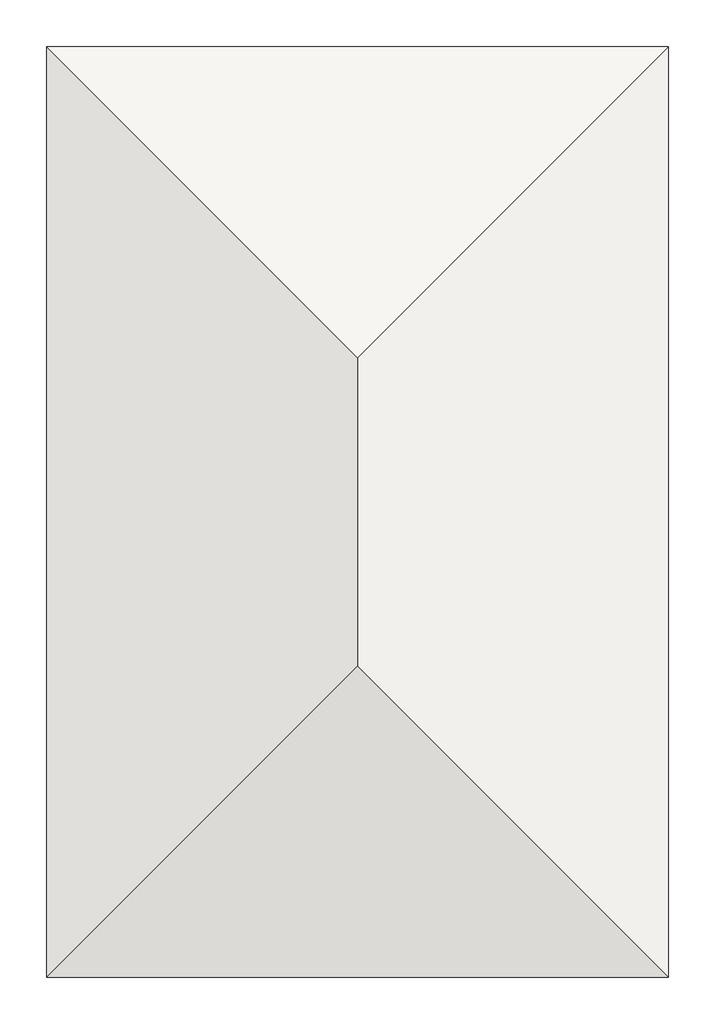
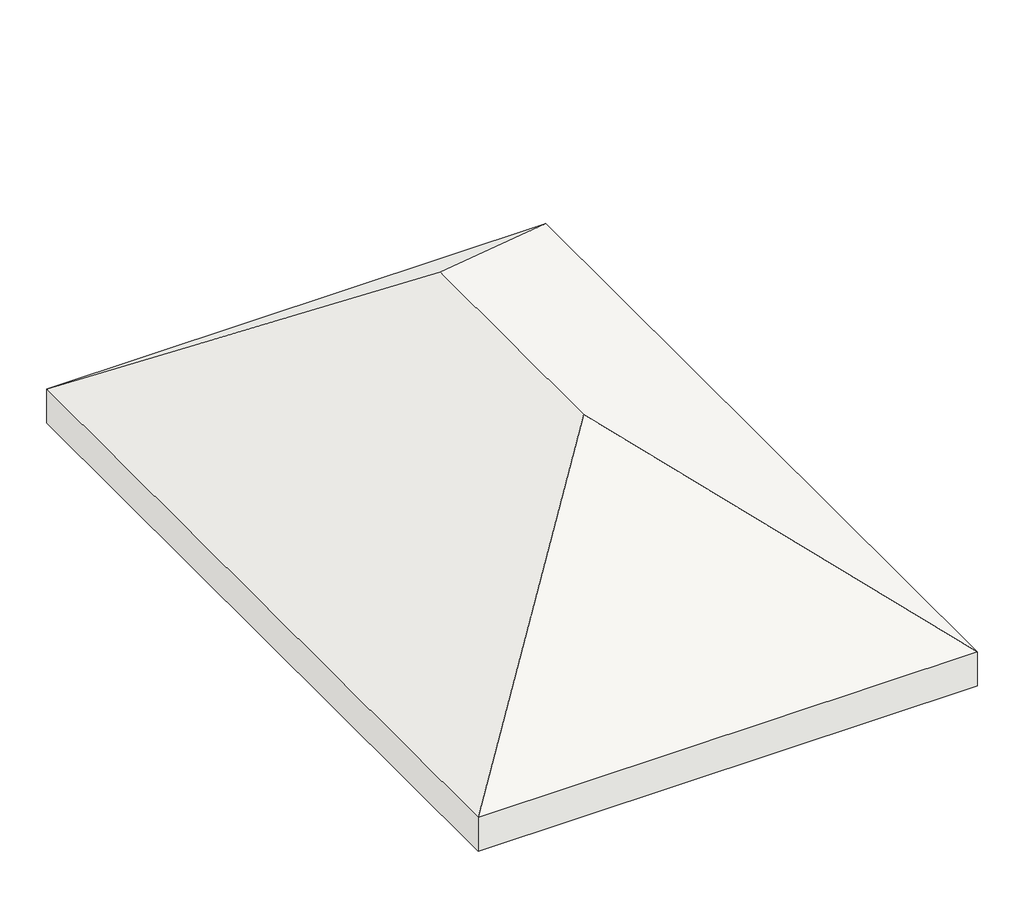
# One storey: 1 roof.
"""IFC4 building model written with IfcOpenShell, lengths in millimetres."""

from ifc_helpers import new_model, si_unit, origin, place, context, project, spatial, faceted_brep, element, save

model = new_model("IFC4")

# Units and contexts
model_context = context("Model", 3, world=origin())
ifc_project = project(units=[si_unit("LENGTHUNIT", "METRE", prefix="MILLI")], contexts=[model_context])

# Site, building, storey
site = spatial("IfcSite", under=ifc_project)
building = spatial("IfcBuilding", under=site)
storey = spatial("IfcBuildingStorey", under=building, Elevation=8686.8)

# Roof
placement = place(None, origin())
element("IfcRoof", 1, ObjectType="slab 1 6\"", at=placement, inside=storey, context=model_context, shape_type="Brep", body=[
    faceted_brep([(-10859.7771954, -5303.8552609, 8686.8), (-9538.9771954, -3983.0552609, 9677.4), (-8218.1771954, -5303.8552609, 8686.8), (-9538.9771954, -2671.4727897, 9677.4), (-8218.1771954, -1350.6727897, 8686.8), (-10859.7771954, -1350.6727897, 8686.8), (-10859.7771954, -5303.8552609, 8877.3), (-8218.1771954, -5303.8552609, 8877.3), (-9538.9771954, -3983.0552609, 9867.9), (-8218.1771954, -1350.6727897, 8877.3), (-9538.9771954, -2671.4727897, 9867.9), (-10859.7771954, -1350.6727897, 8877.3)], [[[0, 1, 2]], [[2, 1, 3, 4]], [[4, 3, 5]], [[1, 0, 5, 3]], [[6, 7, 8]], [[7, 9, 10, 8]], [[9, 11, 10]], [[6, 8, 10, 11]], [[2, 7, 6, 0]], [[4, 9, 7, 2]], [[5, 11, 9, 4]], [[0, 6, 11, 5]]]),
])

save(model, "model.ifc")

# Revit data of these elements
# Type "slab 1 6\""
#   Assembly Code = "B1020"
#   Layers, outside or top first: 0' - 6" "slab colour" (function 1)
# Element 1 (IfcRoof, "slab 1 6\"")
#   built-in parameter 1001705 = 32.375 (stored number, unit not read)
#   built-in parameter 1001710 = 33615
#   Phase Created = New Construction
#   Materials on its faces: "slab colour"
# Materials
#   "slab colour": class "Generic", colour RGB 120 120 120, transparency 0, Cost = 0
